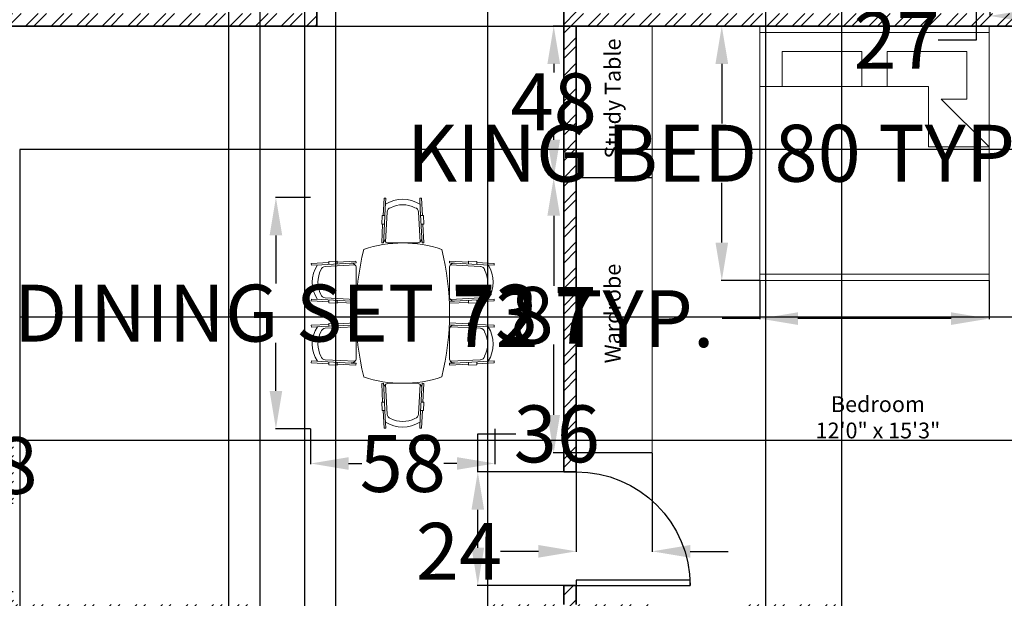
# Model space of a CAD drawing. Units: inches. Extents: x 7 to 752, y -275 to 426.
# Tile 3 of 5: x 284 to 596, y -46 to 137. Entities that reach past the tile are written whole.
import ezdxf

# ---------------------------------------------------------------- set-up
doc = ezdxf.new("R2010")
doc.units = ezdxf.units.IN
for name, color, linetype, lineweight in [('A-ANNO-DIMS', 2, 'Continuous', 18), ('A-ANNO-TEXT', 7, 'Continuous', 18), ('A-AREA-IDEN', 7, 'Continuous', 18), ('A-DOOR', 6, 'Continuous', 25), ('A-FLOR-CASE', 2, 'Continuous', 18), ('A-WALL-PATT', 252, 'Continuous', 13), ('Furniture', 2, 'Continuous', 18), ('Inner Wall', 5, 'Continuous', 35)]:
    doc.layers.add(name, color=color, linetype=linetype, lineweight=lineweight)
doc.styles.get("Standard").update_dxf_attribs({"font": 'arial.ttf'})
doc.dimstyles.get("Standard").update_dxf_attribs({"dimtxt": 18, "dimasz": 12, "dimexe": 0.18, "dimexo": 0.0625, "dimgap": 0.09, "dimtad": 0, "dimtih": 1, "dimtoh": 1, "dimdec": 0, "dimzin": 0, "dimdsep": 46, "dimlunit": 3, "dimtxsty": 'Standard', "dimcen": 0.09, "dimadec": 0, "dimazin": 0, "dimtfac": 1, "dimtdec": 0, "dimtofl": 0, "dimtmove": 0, "dimatfit": 3, "dimfxl": 1, "dimtolj": 1, "dimtzin": 0, "dimarcsym": 0})

# ---------------------------------------------------------------- blocks, each defined once
blk = doc.blocks.new('*U3')
for p, q in [((0, 0), (0, -4)), ((36, 0), (36, -4))]:
    blk.add_line(p, q)
blk.add_lwpolyline([(0, 0), (0, 36), (1.75, 36), (1.75, 0)], close=True)
blk.add_arc((0, 0), 36, 0, 90)
blk = doc.blocks.new('A$C6BEF12A9')
for p, q in [((0.698, 1.955), (0.688, 1.768)), ((0.698, 1.955), (0.718, 1.954)), ((0.718, 1.954), (0.712, 1.841)), ((1.099, 1.955), (1.079, 1.954)), ((1.079, 1.954), (1.085, 1.841)), ((1.099, 1.955), (1.109, 1.768)), ((1.358, 1.955), (1.349, 1.768)), ((1.358, 1.955), (1.378, 1.954)), ((1.378, 1.954), (1.372, 1.841)), ((1.76, 1.955), (1.74, 1.954)), ((1.74, 1.954), (1.746, 1.841)), ((1.76, 1.955), (1.77, 1.768)), ((0.712, 1.841), (0.695, 1.529)), ((0.712, 1.841), (0.695, 1.529)), ((0.73, 1.806), (0.713, 1.488)), ((1.067, 1.806), (1.084, 1.488)), ((1.085, 1.841), (1.102, 1.529)), ((1.372, 1.841), (1.356, 1.529)), ((1.372, 1.841), (1.356, 1.529)), ((1.391, 1.806), (1.374, 1.488)), ((1.728, 1.806), (1.744, 1.488)), ((1.746, 1.841), (1.762, 1.529)), ((0.678, 1.768), (0.673, 1.678)), ((0.708, 1.768), (0.678, 1.768)), ((1.089, 1.768), (1.119, 1.768)), ((1.119, 1.768), (1.124, 1.678)), ((1.339, 1.768), (1.334, 1.678)), ((1.369, 1.768), (1.339, 1.768)), ((1.75, 1.768), (1.78, 1.768)), ((1.78, 1.768), (1.784, 1.678)), ((0.683, 1.678), (0.673, 1.477)), ((0.703, 1.678), (0.673, 1.678)), ((1.094, 1.678), (1.124, 1.678)), ((1.114, 1.678), (1.124, 1.477)), ((1.344, 1.678), (1.333, 1.477)), ((1.364, 1.678), (1.334, 1.678)), ((1.754, 1.678), (1.784, 1.678)), ((1.774, 1.678), (1.785, 1.477)), ((0.673, 1.477), (0.693, 1.476)), ((0.693, 1.476), (0.695, 1.526)), ((0.745, 1.476), (1.052, 1.476)), ((1.104, 1.476), (1.102, 1.526)), ((1.124, 1.477), (1.104, 1.476)), ((1.333, 1.477), (1.353, 1.476)), ((1.353, 1.476), (1.356, 1.526)), ((1.406, 1.476), (1.712, 1.476)), ((1.765, 1.476), (1.762, 1.526)), ((1.785, 1.477), (1.765, 1.476)), ((0, 1.178), (0.187, 1.188)), ((0, 1.178), (0.001, 1.158)), ((0.001, 1.158), (0.114, 1.164)), ((0.114, 1.164), (0.426, 1.181)), ((0.149, 1.146), (0.467, 1.163)), ((0.187, 1.198), (0.277, 1.203)), ((0.187, 1.168), (0.187, 1.198)), ((0.277, 1.193), (0.477, 1.203)), ((0.277, 1.173), (0.277, 1.203)), ((0.479, 1.183), (0.429, 1.181)), ((0.477, 1.203), (0.479, 1.183)), ((1.98, 1.203), (1.979, 1.183)), ((1.979, 1.183), (2.029, 1.181)), ((2.18, 1.193), (1.98, 1.203)), ((2.309, 1.146), (1.99, 1.163)), ((2.343, 1.164), (2.031, 1.181)), ((2.18, 1.173), (2.18, 1.203)), ((2.27, 1.198), (2.18, 1.203)), ((2.27, 1.168), (2.27, 1.198)), ((2.458, 1.178), (2.27, 1.188)), ((2.457, 1.158), (2.343, 1.164)), ((2.458, 1.178), (2.457, 1.158)), ((0.479, 0.824), (0.479, 1.131)), ((1.979, 0.824), (1.979, 1.131)), ((0, 0.777), (0.001, 0.797)), ((0, 0.777), (0.187, 0.767)), ((0.001, 0.797), (0.114, 0.791)), ((0.114, 0.791), (0.426, 0.774)), ((0.114, 0.791), (0.426, 0.774)), ((0.149, 0.809), (0.467, 0.792)), ((0.187, 0.787), (0.187, 0.757)), ((0.187, 0.757), (0.277, 0.752)), ((0.277, 0.782), (0.277, 0.752)), ((0.277, 0.762), (0.477, 0.752)), ((0.479, 0.772), (0.429, 0.774)), ((0.477, 0.752), (0.479, 0.772)), ((1.979, 0.772), (2.029, 0.774)), ((1.98, 0.752), (1.979, 0.772)), ((2.18, 0.762), (1.98, 0.752)), ((2.309, 0.809), (1.99, 0.792)), ((2.343, 0.791), (2.031, 0.774)), ((2.343, 0.791), (2.031, 0.774)), ((2.18, 0.782), (2.18, 0.752)), ((2.27, 0.757), (2.18, 0.752)), ((2.27, 0.787), (2.27, 0.757)), ((2.458, 0.777), (2.27, 0.767)), ((2.457, 0.797), (2.343, 0.791)), ((2.458, 0.777), (2.457, 0.797)), ((0.673, 0.477), (0.693, 0.479)), ((0.683, 0.277), (0.673, 0.477)), ((0.693, 0.479), (0.695, 0.429)), ((0.712, 0.114), (0.695, 0.426)), ((0.712, 0.114), (0.695, 0.426)), ((0.73, 0.149), (0.713, 0.467)), ((0.745, 0.479), (1.052, 0.479)), ((1.067, 0.149), (1.084, 0.467)), ((1.085, 0.114), (1.102, 0.426)), ((1.104, 0.479), (1.102, 0.429)), ((1.124, 0.477), (1.104, 0.479)), ((1.114, 0.277), (1.124, 0.477)), ((1.333, 0.477), (1.353, 0.479)), ((1.344, 0.277), (1.333, 0.477)), ((1.353, 0.479), (1.356, 0.429)), ((1.372, 0.114), (1.356, 0.426)), ((1.372, 0.114), (1.356, 0.426)), ((1.391, 0.149), (1.374, 0.467)), ((1.406, 0.479), (1.712, 0.479)), ((1.728, 0.149), (1.744, 0.467)), ((1.746, 0.114), (1.762, 0.426)), ((1.765, 0.479), (1.762, 0.429)), ((1.785, 0.477), (1.765, 0.479)), ((1.774, 0.277), (1.785, 0.477)), ((0.678, 0.187), (0.673, 0.277)), ((0.703, 0.277), (0.673, 0.277)), ((1.094, 0.277), (1.124, 0.277)), ((1.119, 0.187), (1.124, 0.277)), ((1.364, 0.277), (1.334, 0.277)), ((1.339, 0.187), (1.334, 0.277)), ((1.754, 0.277), (1.784, 0.277)), ((1.78, 0.187), (1.784, 0.277)), ((0.708, 0.187), (0.678, 0.187)), ((0.698, 0), (0.688, 0.187)), ((0.718, 0.001), (0.712, 0.114)), ((1.079, 0.001), (1.085, 0.114)), ((1.089, 0.187), (1.119, 0.187)), ((1.099, 0), (1.109, 0.187)), ((1.369, 0.187), (1.339, 0.187)), ((1.358, 0), (1.349, 0.187)), ((1.378, 0.001), (1.372, 0.114)), ((1.74, 0.001), (1.746, 0.114)), ((1.75, 0.187), (1.78, 0.187)), ((1.76, 0), (1.77, 0.187)), ((0.698, 0), (0.718, 0.001)), ((1.099, 0), (1.079, 0.001)), ((1.358, 0), (1.378, 0.001)), ((1.76, 0), (1.74, 0.001))]:
    blk.add_line(p, q)
for centre, radius, start, end in [((0.898, 1.603), 0.341, 57.3412, 122.6588), ((1.559, 1.603), 0.341, 57.3412, 122.6588), ((0.78, 1.804), 0.05, 103.7138, 177), ((0.898, 1.603), 0.281, 62.3651, 117.6349), ((1.017, 1.804), 0.05, 3, 76.2862), ((1.441, 1.804), 0.05, 103.7138, 177), ((1.559, 1.603), 0.281, 62.3651, 117.6349), ((1.678, 1.804), 0.05, 3, 76.2862), ((1.229, -1.385), 2.862, 76.2365, 103.7635), ((0.745, 1.526), 0.05, 177, 270), ((1.052, 1.526), 0.05, 270, 3), ((1.406, 1.526), 0.05, 177, 270), ((1.712, 1.526), 0.05, 270, 3), ((1.779, 0.977), 1.3, 161.253, 198.747), ((0.679, 0.977), 1.3, 341.253, 18.747), ((0.352, 0.977), 0.341, 147.3412, 212.6588), ((0.429, 1.131), 0.05, 0, 93), ((2.029, 1.131), 0.05, 87, 180), ((2.106, 0.977), 0.341, 327.3412, 32.6588), ((0.352, 0.977), 0.281, 152.3651, 207.6349), ((0.151, 1.096), 0.05, 93, 166.2862), ((2.306, 1.096), 0.05, 13.7138, 87), ((2.106, 0.977), 0.281, 332.3651, 27.6349), ((0.151, 0.859), 0.05, 193.7138, 267), ((2.306, 0.859), 0.05, 273, 346.2862), ((0.429, 0.824), 0.05, 267, 0), ((2.029, 0.824), 0.05, 180, 273), ((1.229, 3.34), 2.862, 256.2365, 283.7635), ((0.745, 0.429), 0.05, 90, 183), ((1.052, 0.429), 0.05, 357, 90), ((1.406, 0.429), 0.05, 90, 183), ((1.712, 0.429), 0.05, 357, 90), ((0.78, 0.151), 0.05, 183, 256.2862), ((1.017, 0.151), 0.05, 283.7138, 357), ((1.441, 0.151), 0.05, 183, 256.2862), ((1.678, 0.151), 0.05, 283.7138, 357), ((0.898, 0.352), 0.341, 237.3412, 302.6588), ((0.898, 0.352), 0.281, 242.3651, 297.6349), ((1.559, 0.352), 0.341, 237.3412, 302.6588), ((1.559, 0.352), 0.281, 242.3651, 297.6349)]:
    blk.add_arc(centre, radius, start, end)
blk = doc.blocks.new('KING-00')
for p, q in [((-0.8967, -0.947), (-0.8967, 0.8818)), ((0.6019, 0.8818), (0.6019, -0.4644)), ((1.0337, -0.947), (1.0337, 0.8818)), ((0.6019, 0.704), (0.8813, 0.704)), ((0.8813, 0.069), (0.8813, 0.704)), ((0.6019, 0.069), (0.8813, 0.069)), ((0.8813, -0.1342), (0.6019, -0.1342)), ((0.8813, -0.7692), (0.8813, -0.1342)), ((0.1193, -0.4644), (0.1193, -0.947)), ((0.6019, -0.4644), (0.1193, -0.4644)), ((0.1193, -0.947), (0.5003, -0.566)), ((0.5003, -0.7692), (0.5003, -0.566)), ((0.5003, -0.7692), (0.8813, -0.7692))]:
    blk.add_line(p, q)
blk.add_lwpolyline([(-0.9475, -0.947), (-0.9475, 0.8818), (1.0845, 0.8818), (1.0845, -0.947)], close=True)
blk = doc.blocks.new('*D20')
at = {"layer": 'A-ANNO-DIMS', "color": 0, "lineweight": -2, "transparency": 16777216}
for p, q in [((518.33, 134.68), (506.15, 134.68)), ((506.33, 122.68), (506.33, 103.84)), ((506.33, 66.2), (506.33, 85.04)), ((518.33, 54.2), (506.15, 54.2))]:
    blk.add_line(p, q, dxfattribs=at)
at = {"layer": 'A-ANNO-DIMS', "color": 0, "transparency": 16777216}
for points in [[(504.33, 122.68), (508.33, 122.68), (506.33, 134.68)], [(504.33, 66.2), (508.33, 66.2), (506.33, 54.2)]]:
    blk.add_solid(points, dxfattribs=at)
at = {"layer": 'Defpoints', "color": 0, "transparency": 16777216}
for p in [(506.33, 134.68), (518.4, 134.68), (518.4, 54.2)]:
    blk.add_point(p, dxfattribs=at)
at = {"layer": 'A-ANNO-DIMS', "color": 0, "transparency": 16777216, "insert": (506.33, 94.44), "char_height": 18, "attachment_point": 5}
blk.add_mtext('\\A1;KING BED 80 TYP.', dxfattribs=at)
blk = doc.blocks.new('*D21')
at = {"layer": 'A-ANNO-DIMS', "color": 0, "lineweight": -2, "transparency": 16777216}
for p, q in [((518.4, 54.14), (518.4, 41.95)), ((590.82, 54.14), (590.82, 41.95)), ((518.4, 42.13), (506.4, 42.13)), ((578.82, 42.13), (530.4, 42.13))]:
    blk.add_line(p, q, dxfattribs=at)
at = {"layer": 'A-ANNO-DIMS', "color": 0, "transparency": 16777216}
for points in [[(530.4, 44.13), (530.4, 40.13), (518.4, 42.13)], [(578.82, 44.13), (578.82, 40.13), (590.82, 42.13)]]:
    blk.add_solid(points, dxfattribs=at)
at = {"layer": 'Defpoints', "color": 0, "transparency": 16777216}
for p in [(518.4, 54.2), (590.82, 54.2), (518.4, 42.13)]:
    blk.add_point(p, dxfattribs=at)
at = {"layer": 'A-ANNO-DIMS', "color": 0, "transparency": 16777216, "insert": (462.57, 42.13), "char_height": 18, "attachment_point": 5}
blk.add_mtext('\\A1;72 TYP.', dxfattribs=at)
blk = doc.blocks.new('*D22')
at = {"layer": 'A-ANNO-DIMS', "color": 0, "lineweight": -2, "transparency": 16777216}
for p, q in [((376.25, 80.45), (365.16, 80.45)), ((365.34, 68.45), (365.34, 53.28)), ((365.34, 19.29), (365.34, 34.47)), ((376.25, 7.29), (365.16, 7.29))]:
    blk.add_line(p, q, dxfattribs=at)
at = {"layer": 'A-ANNO-DIMS', "color": 0, "transparency": 16777216}
for points in [[(363.34, 68.45), (367.34, 68.45), (365.34, 80.45)], [(363.34, 19.29), (367.34, 19.29), (365.34, 7.29)]]:
    blk.add_solid(points, dxfattribs=at)
at = {"layer": 'Defpoints', "color": 0, "transparency": 16777216}
for p in [(376.32, 80.45), (365.34, 7.29), (376.32, 7.29)]:
    blk.add_point(p, dxfattribs=at)
at = {"layer": 'A-ANNO-DIMS', "color": 0, "transparency": 16777216, "insert": (365.34, 43.87), "char_height": 18, "attachment_point": 5}
blk.add_mtext('\\A1;DINING SET 73', dxfattribs=at)
blk = doc.blocks.new('*D23')
at = {"layer": 'A-ANNO-DIMS', "color": 0, "lineweight": -2, "transparency": 16777216}
for p, q in [((376.32, 7.23), (376.32, -3.86)), ((434.6, 7.23), (434.6, -3.86)), ((388.32, -3.68), (392.46, -3.68)), ((422.6, -3.68), (418.46, -3.68))]:
    blk.add_line(p, q, dxfattribs=at)
at = {"layer": 'A-ANNO-DIMS', "color": 0, "transparency": 16777216}
for points in [[(388.32, -1.68), (388.32, -5.68), (376.32, -3.68)], [(422.6, -1.68), (422.6, -5.68), (434.6, -3.68)]]:
    blk.add_solid(points, dxfattribs=at)
at = {"layer": 'Defpoints', "color": 0, "transparency": 16777216}
for p in [(376.32, 7.29), (434.6, 7.29), (434.6, -3.68)]:
    blk.add_point(p, dxfattribs=at)
at = {"layer": 'A-ANNO-DIMS', "color": 0, "transparency": 16777216, "insert": (405.46, -3.68), "char_height": 18, "attachment_point": 5}
blk.add_mtext('\\A1;58', dxfattribs=at)
blk = doc.blocks.new('*D26')
at = {"layer": 'A-ANNO-DIMS', "color": 0, "lineweight": -2, "transparency": 16777216}
for p, q in [((591.04, 142.1), (591.04, 137.69)), ((619.61, 142.1), (619.61, 137.69)), ((603.04, 137.87), (607.61, 137.87)), ((619.61, 137.87), (631.61, 137.87))]:
    blk.add_line(p, q, dxfattribs=at)
at = {"layer": 'A-ANNO-DIMS', "color": 0, "transparency": 16777216}
for points in [[(603.04, 139.87), (603.04, 135.87), (591.04, 137.87)], [(607.61, 139.87), (607.61, 135.87), (619.61, 137.87)]]:
    blk.add_solid(points, dxfattribs=at)
at = {"layer": 'Defpoints', "color": 0, "transparency": 16777216}
for p in [(591.04, 142.16), (619.61, 142.16), (619.61, 137.87)]:
    blk.add_point(p, dxfattribs=at)
at = {"layer": 'A-ANNO-DIMS', "color": 0, "transparency": 16777216, "insert": (695.1, 137.87), "char_height": 18, "attachment_point": 5}
blk.add_mtext('\\A1;FRIDGE 29', dxfattribs=at)
blk = doc.blocks.new('*D27')
at = {"layer": 'A-ANNO-DIMS', "color": 0, "lineweight": -2, "transparency": 16777216}
for p, q in [((590.98, 168.83), (586.58, 168.83)), ((586.76, 156.83), (586.76, 154.16)), ((590.98, 142.16), (586.58, 142.16)), ((586.76, 142.16), (586.76, 130.16)), ((586.76, 130.16), (574.76, 130.16))]:
    blk.add_line(p, q, dxfattribs=at)
at = {"layer": 'A-ANNO-DIMS', "color": 0, "transparency": 16777216}
for points in [[(584.76, 156.83), (588.76, 156.83), (586.76, 168.83)], [(584.76, 154.16), (588.76, 154.16), (586.76, 142.16)]]:
    blk.add_solid(points, dxfattribs=at)
at = {"layer": 'Defpoints', "color": 0, "transparency": 16777216}
for p in [(591.04, 168.83), (586.76, 142.16), (591.04, 142.16)]:
    blk.add_point(p, dxfattribs=at)
at = {"layer": 'A-ANNO-DIMS', "color": 0, "transparency": 16777216, "insert": (561.62, 130.16), "char_height": 18, "attachment_point": 5}
blk.add_mtext('\\A1;27', dxfattribs=at)
blk = doc.blocks.new('*D39')
at = {"layer": 'A-ANNO-DIMS', "color": 0, "lineweight": -2, "transparency": 16777216}
for p, q in [((348.33, 413.83), (336.33, 413.83)), ((360.33, -131.26), (360.33, 414.01)), ((384.33, -131.26), (384.33, 414.01)), ((396.33, 413.83), (408.33, 413.83))]:
    blk.add_line(p, q, dxfattribs=at)
at = {"layer": 'A-ANNO-DIMS', "color": 0, "transparency": 16777216}
for points in [[(348.33, 415.83), (348.33, 411.83), (360.33, 413.83)], [(396.33, 415.83), (396.33, 411.83), (384.33, 413.83)]]:
    blk.add_solid(points, dxfattribs=at)
at = {"layer": 'Defpoints', "color": 0, "transparency": 16777216}
for p in [(384.33, 413.83), (360.33, -131.32), (384.33, -131.32)]:
    blk.add_point(p, dxfattribs=at)
at = {"layer": 'A-ANNO-DIMS', "color": 0, "transparency": 16777216, "insert": (421.43, 413.83), "char_height": 18, "attachment_point": 5}
blk.add_mtext('\\A1;24', dxfattribs=at)
blk = doc.blocks.new('*D40')
at = {"layer": 'A-ANNO-DIMS', "color": 0, "lineweight": -2, "transparency": 16777216}
for p, q in [((372.328243, 413.826615), (360.328243, 413.826615)), ((384.328243, -106.961989), (384.328243, 414.006615)), ((432.328243, -106.961989), (432.328243, 414.006615)), ((444.328243, 413.826615), (456.328243, 413.826615))]:
    blk.add_line(p, q, dxfattribs=at)
at = {"layer": 'A-ANNO-DIMS', "color": 0, "transparency": 16777216}
for points in [[(372.328243, 415.826615), (372.328243, 411.826615), (384.328243, 413.826615)], [(444.328243, 415.826615), (444.328243, 411.826615), (432.328243, 413.826615)]]:
    blk.add_solid(points, dxfattribs=at)
at = {"layer": 'Defpoints', "color": 0, "transparency": 16777216}
for p in [(432.328243, 413.826615), (384.328243, -107.024489), (432.328243, -107.024489)]:
    blk.add_point(p, dxfattribs=at)
at = {"layer": 'A-ANNO-DIMS', "color": 0, "transparency": 16777216, "insert": (408.328243, 413.826615), "char_height": 18, "attachment_point": 5}
blk.add_mtext('\\A1;48', dxfattribs=at)
blk = doc.blocks.new('*D42')
at = {"layer": 'A-ANNO-DIMS', "color": 0, "lineweight": -2, "transparency": 16777216}
for p, q in [((221.33, 95.61), (221.33, -259.65)), ((284.33, 95.61), (284.33, -259.65)), ((233.33, -259.47), (239.8, -259.47)), ((272.33, -259.47), (265.86, -259.47))]:
    blk.add_line(p, q, dxfattribs=at)
at = {"layer": 'A-ANNO-DIMS', "color": 0, "transparency": 16777216}
for points in [[(233.33, -257.47), (233.33, -261.47), (221.33, -259.47)], [(272.33, -257.47), (272.33, -261.47), (284.33, -259.47)]]:
    blk.add_solid(points, dxfattribs=at)
at = {"layer": 'Defpoints', "color": 0, "transparency": 16777216}
for p in [(221.33, 95.68), (284.33, 95.68), (284.33, -259.47)]:
    blk.add_point(p, dxfattribs=at)
at = {"layer": 'A-ANNO-DIMS', "color": 0, "transparency": 16777216, "insert": (252.83, -259.47), "char_height": 18, "attachment_point": 5}
blk.add_mtext('\\A1;63', dxfattribs=at)
blk = doc.blocks.new('*D43')
at = {"layer": 'A-ANNO-DIMS', "color": 0, "lineweight": -2, "transparency": 16777216}
for p, q in [((221.39, 134.68), (657.66, 134.68)), ((657.48, 122.68), (657.48, 78.46)), ((657.48, 15.68), (657.48, 59.89)), ((221.39, 3.68), (657.66, 3.68))]:
    blk.add_line(p, q, dxfattribs=at)
at = {"layer": 'A-ANNO-DIMS', "color": 0, "transparency": 16777216}
for points in [[(655.48, 122.68), (659.48, 122.68), (657.48, 134.68)], [(655.48, 15.68), (659.48, 15.68), (657.48, 3.68)]]:
    blk.add_solid(points, dxfattribs=at)
at = {"layer": 'Defpoints', "color": 0, "transparency": 16777216}
for p in [(221.33, 134.68), (657.48, 134.68), (221.33, 3.68)]:
    blk.add_point(p, dxfattribs=at)
at = {"layer": 'A-ANNO-DIMS', "color": 0, "transparency": 16777216, "insert": (657.48, 69.18), "char_height": 18, "attachment_point": 5}
blk.add_mtext('\\A1;131', dxfattribs=at)
blk = doc.blocks.new('*D44')
at = {"layer": 'A-ANNO-DIMS', "color": 0, "lineweight": -2, "transparency": 16777216}
for p, q in [((657.48, 42.68), (657.48, 54.68)), ((657.48, 54.68), (669.48, 54.68)), ((284.39, 42.68), (657.66, 42.68)), ((657.48, 15.68), (657.48, 30.68)), ((284.39, 3.68), (657.66, 3.68))]:
    blk.add_line(p, q, dxfattribs=at)
at = {"layer": 'A-ANNO-DIMS', "color": 0, "transparency": 16777216}
for points in [[(655.48, 30.68), (659.48, 30.68), (657.48, 42.68)], [(655.48, 15.68), (659.48, 15.68), (657.48, 3.68)]]:
    blk.add_solid(points, dxfattribs=at)
at = {"layer": 'Defpoints', "color": 0, "transparency": 16777216}
for p in [(284.33, 42.68), (657.48, 42.68), (284.33, 3.68)]:
    blk.add_point(p, dxfattribs=at)
at = {"layer": 'A-ANNO-DIMS', "color": 0, "transparency": 16777216, "insert": (682.47, 54.68), "char_height": 18, "attachment_point": 5}
blk.add_mtext('\\A1;39', dxfattribs=at)
blk = doc.blocks.new('*D45')
at = {"layer": 'A-ANNO-DIMS', "color": 0, "lineweight": -2, "transparency": 16777216}
for p, q in [((284.39, 95.68), (657.66, 95.68)), ((657.48, 83.68), (657.48, 78.46)), ((657.48, 54.68), (657.48, 59.89)), ((284.39, 42.68), (657.66, 42.68))]:
    blk.add_line(p, q, dxfattribs=at)
at = {"layer": 'A-ANNO-DIMS', "color": 0, "transparency": 16777216}
for points in [[(655.48, 83.68), (659.48, 83.68), (657.48, 95.68)], [(655.48, 54.68), (659.48, 54.68), (657.48, 42.68)]]:
    blk.add_solid(points, dxfattribs=at)
at = {"layer": 'Defpoints', "color": 0, "transparency": 16777216}
for p in [(284.33, 95.68), (657.48, 95.68), (284.33, 42.68)]:
    blk.add_point(p, dxfattribs=at)
at = {"layer": 'A-ANNO-DIMS', "color": 0, "transparency": 16777216, "insert": (657.48, 69.18), "char_height": 18, "attachment_point": 5}
blk.add_mtext('\\A1;53', dxfattribs=at)
blk = doc.blocks.new('*D46')
at = {"layer": 'A-ANNO-DIMS', "color": 0, "lineweight": -2, "transparency": 16777216}
for p, q in [((520.16, 197.44), (520.16, -259.65)), ((544.16, 197.44), (544.16, -259.65)), ((508.16, -259.47), (496.16, -259.47)), ((556.16, -259.47), (568.16, -259.47))]:
    blk.add_line(p, q, dxfattribs=at)
at = {"layer": 'A-ANNO-DIMS', "color": 0, "transparency": 16777216}
for points in [[(508.16, -257.47), (508.16, -261.47), (520.16, -259.47)], [(556.16, -257.47), (556.16, -261.47), (544.16, -259.47)]]:
    blk.add_solid(points, dxfattribs=at)
at = {"layer": 'Defpoints', "color": 0, "transparency": 16777216}
for p in [(520.16, 197.5), (544.16, 197.5), (544.16, -259.47)]:
    blk.add_point(p, dxfattribs=at)
at = {"layer": 'A-ANNO-DIMS', "color": 0, "transparency": 16777216, "insert": (581.26, -259.47), "char_height": 18, "attachment_point": 5}
blk.add_mtext('\\A1;24', dxfattribs=at)
blk = doc.blocks.new('*D52')
at = {"layer": 'A-ANNO-DIMS', "color": 0, "lineweight": -2, "transparency": 16777216}
for p, q in [((350.33, 198.78), (350.33, -259.65)), ((374.33, 198.78), (374.33, -259.65)), ((338.33, -259.47), (326.33, -259.47)), ((386.33, -259.47), (398.33, -259.47))]:
    blk.add_line(p, q, dxfattribs=at)
at = {"layer": 'A-ANNO-DIMS', "color": 0, "transparency": 16777216}
for points in [[(338.33, -257.47), (338.33, -261.47), (350.33, -259.47)], [(386.33, -257.47), (386.33, -261.47), (374.33, -259.47)]]:
    blk.add_solid(points, dxfattribs=at)
at = {"layer": 'Defpoints', "color": 0, "transparency": 16777216}
for p in [(350.33, 198.85), (374.33, 198.85), (374.33, -259.47)]:
    blk.add_point(p, dxfattribs=at)
at = {"layer": 'A-ANNO-DIMS', "color": 0, "transparency": 16777216, "insert": (411.43, -259.47), "char_height": 18, "attachment_point": 5}
blk.add_mtext('\\A1;24', dxfattribs=at)
blk = doc.blocks.new('*D55')
at = {"layer": 'A-ANNO-DIMS', "color": 0, "lineweight": -2, "transparency": 16777216}
for p, q in [((429.18, -6.32), (429.18, 5.68)), ((429.18, 5.68), (441.18, 5.68)), ((460.27, -6.32), (429, -6.32)), ((429.18, -30.32), (429.18, -18.32)), ((460.27, -42.32), (429, -42.32))]:
    blk.add_line(p, q, dxfattribs=at)
at = {"layer": 'A-ANNO-DIMS', "color": 0, "transparency": 16777216}
for points in [[(427.18, -18.32), (431.18, -18.32), (429.18, -6.32)], [(427.18, -30.32), (431.18, -30.32), (429.18, -42.32)]]:
    blk.add_solid(points, dxfattribs=at)
at = {"layer": 'Defpoints', "color": 0, "transparency": 16777216}
for p in [(429.18, -6.32), (460.33, -6.32), (460.33, -42.32)]:
    blk.add_point(p, dxfattribs=at)
at = {"layer": 'A-ANNO-DIMS', "color": 0, "transparency": 16777216, "insert": (454.15, 5.68), "char_height": 18, "attachment_point": 5}
blk.add_mtext('\\A1;36', dxfattribs=at)
blk = doc.blocks.new('*D57')
at = {"layer": 'A-ANNO-DIMS', "color": 0, "lineweight": -2, "transparency": 16777216}
for p, q in [((460.33, -0.39), (460.33, -31.65)), ((484.33, -0.39), (484.33, -31.65)), ((448.33, -31.47), (436.33, -31.47)), ((496.33, -31.47), (508.33, -31.47))]:
    blk.add_line(p, q, dxfattribs=at)
at = {"layer": 'A-ANNO-DIMS', "color": 0, "transparency": 16777216}
for points in [[(448.33, -29.47), (448.33, -33.47), (460.33, -31.47)], [(496.33, -29.47), (496.33, -33.47), (484.33, -31.47)]]:
    blk.add_solid(points, dxfattribs=at)
at = {"layer": 'Defpoints', "color": 0, "transparency": 16777216}
for p in [(460.33, -0.32), (484.33, -0.32), (460.33, -31.47)]:
    blk.add_point(p, dxfattribs=at)
at = {"layer": 'A-ANNO-DIMS', "color": 0, "transparency": 16777216, "insert": (423.23, -31.47), "char_height": 18, "attachment_point": 5}
blk.add_mtext('\\A1;24', dxfattribs=at)
blk = doc.blocks.new('*D58')
at = {"layer": 'A-ANNO-DIMS', "color": 0, "lineweight": -2, "transparency": 16777216}
for p, q in [((484.27, 86.68), (453, 86.68)), ((453.18, 74.68), (453.18, 52.46)), ((453.18, 11.68), (453.18, 33.9)), ((484.27, -0.32), (453, -0.32))]:
    blk.add_line(p, q, dxfattribs=at)
at = {"layer": 'A-ANNO-DIMS', "color": 0, "transparency": 16777216}
for points in [[(451.18, 74.68), (455.18, 74.68), (453.18, 86.68)], [(451.18, 11.68), (455.18, 11.68), (453.18, -0.32)]]:
    blk.add_solid(points, dxfattribs=at)
at = {"layer": 'Defpoints', "color": 0, "transparency": 16777216}
for p in [(453.18, 86.68), (484.33, 86.68), (484.33, -0.32)]:
    blk.add_point(p, dxfattribs=at)
at = {"layer": 'A-ANNO-DIMS', "color": 0, "transparency": 16777216, "insert": (453.18, 43.18), "char_height": 18, "attachment_point": 5}
blk.add_mtext('\\A1;87', dxfattribs=at)
blk = doc.blocks.new('*D59')
at = {"layer": 'A-ANNO-DIMS', "color": 0, "lineweight": -2, "transparency": 16777216}
for p, q in [((484.27, 134.68), (453, 134.68)), ((453.18, 122.68), (453.18, 119.96)), ((453.18, 98.68), (453.18, 101.4)), ((484.27, 86.68), (453, 86.68))]:
    blk.add_line(p, q, dxfattribs=at)
at = {"layer": 'A-ANNO-DIMS', "color": 0, "transparency": 16777216}
for points in [[(451.18, 122.68), (455.18, 122.68), (453.18, 134.68)], [(451.18, 98.68), (455.18, 98.68), (453.18, 86.68)]]:
    blk.add_solid(points, dxfattribs=at)
at = {"layer": 'Defpoints', "color": 0, "transparency": 16777216}
for p in [(453.18, 134.68), (484.33, 134.68), (484.33, 86.68)]:
    blk.add_point(p, dxfattribs=at)
at = {"layer": 'A-ANNO-DIMS', "color": 0, "transparency": 16777216, "insert": (453.18, 110.68), "char_height": 18, "attachment_point": 5}
blk.add_mtext('\\A1;48', dxfattribs=at)
blk = doc.blocks.new('*D63')
at = {"layer": 'A-ANNO-DIMS', "color": 0, "lineweight": -2, "transparency": 16777216}
for p, q in [((251.18, -16.32), (251.18, -4.32)), ((251.18, -4.32), (263.18, -4.32)), ((282.27, -16.32), (251, -16.32)), ((251.18, -32.32), (251.18, -28.32)), ((282.27, -44.32), (251, -44.32))]:
    blk.add_line(p, q, dxfattribs=at)
at = {"layer": 'A-ANNO-DIMS', "color": 0, "transparency": 16777216}
for points in [[(249.18, -28.32), (253.18, -28.32), (251.18, -16.32)], [(249.18, -32.32), (253.18, -32.32), (251.18, -44.32)]]:
    blk.add_solid(points, dxfattribs=at)
at = {"layer": 'Defpoints', "color": 0, "transparency": 16777216}
for p in [(251.18, -16.32), (282.33, -16.32), (282.33, -44.32)]:
    blk.add_point(p, dxfattribs=at)
at = {"layer": 'A-ANNO-DIMS', "color": 0, "transparency": 16777216, "insert": (276.33, -4.32), "char_height": 18, "attachment_point": 5}
blk.add_mtext('\\A1;28', dxfattribs=at)

msp = doc.modelspace()

# ---------------------------------------------------------------- hatches: boundary and pattern name
at = {"layer": 'A-WALL-PATT'}
h = msp.add_hatch(dxfattribs=at)
h.set_pattern_fill('ANSI32', color=256, scale=0.6)
h.set_pattern_definition([(45, (-434.707, -1257.0093), (-4.041115, 4.041115), []), (45, (-432.013, -1257.0093), (-4.041115, 4.041115), [])])
h.paths.add_polyline_path([(360.33, -48.32), (282.33, -48.32), (282.33, -44.32), (278.33, -44.32), (278.33, -48.32), (182.33, -48.32), (182.33, -54.32), (356.33, -54.32), (356.33, -89.32), (360.33, -89.32)])
h.paths.add_polyline_path([(484.33, -48.32), (460.33, -48.32), (460.33, -42.32), (456.33, -42.32), (456.33, -48.32), (432.33, -48.32), (432.33, -52.32), (456.33, -52.32), (456.33, -131.32), (460.33, -131.32), (460.33, -52.32), (484.33, -52.32)])
h.paths.add_polyline_path([(544.33, -48.32), (512.33, -48.32), (512.33, -52.32), (544.33, -52.32)])
h.paths.add_polyline_path([(460.33, 134.68), (484.33, 134.68), (620.33, 134.68), (620.33, 138.68), (460.33, 138.68), (460.33, 144.68), (456.33, 144.68), (456.33, -6.32), (460.33, -6.32)])
h.paths.add_polyline_path([(282.33, 3.68), (182.33, 3.68), (182.33, -0.32), (278.33, -0.32), (278.33, -16.32), (282.33, -16.32)])
h.paths.add_polyline_path([(378.33, 144.68), (374.33, 144.68), (374.33, 138.68), (182.33, 138.68), (182.33, 134.68), (378.33, 134.68)])
h.paths.add_polyline_path([(284.33, 306.68), (278.33, 306.68), (278.33, 286.68), (240.33, 286.68), (240.33, 282.68), (284.33, 282.68)])
h.paths.add_polyline_path([(212.33, 286.68), (182.33, 286.68), (182.33, 282.68), (212.33, 282.68)])
h.paths.add_polyline_path([(436.33, 225.08), (460.33, 225.08), (460.33, 229.08), (432.33, 229.08), (432.33, 184.68), (456.33, 184.68), (456.33, 180.68), (460.33, 180.68), (460.33, 188.68), (436.33, 188.68)])
h.paths.add_polyline_path([(432.33, 204.68), (378.33, 204.68), (378.33, 306.68), (374.33, 306.68), (374.33, 282.68), (374.33, 198.85), (374.33, 180.68), (378.33, 180.68), (378.33, 200.68), (432.33, 200.68)])
h.paths.add_polyline_path([(460.33, 270.68), (436.33, 270.68), (436.33, 306.68), (432.33, 306.68), (432.33, 282.68), (432.33, 266.68), (460.33, 266.68)])

# ---------------------------------------------------------------- linework, layer by layer
at = {"layer": 'A-FLOR-CASE'}
for points in [[(460.33, 134.68), (484.33, 134.68), (484.33, 86.68), (460.33, 86.68)], [(460.33, 86.68), (484.33, 86.68), (484.33, -0.32), (460.33, -0.32)]]:
    msp.add_lwpolyline(points, close=True, dxfattribs=at)
at = {"layer": 'Inner Wall'}
for p, q in [((378.33, 144.68), (378.33, 134.68)), ((456.33, 144.68), (456.33, -6.32)), ((182.33, 134.68), (378.33, 134.68)), ((460.33, 134.68), (620.33, 134.68)), ((460.33, 134.68), (460.33, -6.32)), ((456.33, -6.32), (460.33, -6.32)), ((456.33, -42.32), (460.33, -42.32)), ((456.33, -42.32), (456.33, -48.32)), ((460.33, -42.32), (460.33, -48.32))]:
    msp.add_line(p, q, dxfattribs=at)

# ---------------------------------------------------------------- block references
at = {"layer": 'A-DOOR', "xscale": -1, "rotation": 270}
msp.add_blockref('*U3', (460.33, -42.32), dxfattribs=at)
at = {"layer": 'Furniture'}
for name, p, xscale, yscale, zscale, rotation in [('KING-00', (553.32, 91.73), 39.60249106241186, 39.60249106241186, 39.60249106241186, 90), ('A$C6BEF12A9', (376.53, 80.24), 29.59247402267948, 29.59247402267948, 29.59247402267948, 270)]:
    msp.add_blockref(name, p, dxfattribs=dict(at, xscale=xscale, yscale=yscale, zscale=zscale, rotation=rotation))

# ---------------------------------------------------------------- texts
at = {"layer": 'A-ANNO-TEXT', "char_height": 5, "attachment_point": 3, "rotation": 90}
for s, insert in [('\\pxqc;{\\fTimes New Roman|b0|i0|c0|p18;Study Table}', (469.34, 136.29)), ('\\pxqc;{\\fTimes New Roman|b0|i0|c0|p18;Wardrobe}', (469.34, 68.29))]:
    msp.add_mtext_dynamic_manual_height_columns(s, width=49.1019, gutter_width=12.5, heights=[0], dxfattribs=dict(at, insert=insert))
at = {"layer": 'A-AREA-IDEN', "insert": (580.25, 17.59), "char_height": 5, "attachment_point": 3}
msp.add_mtext_dynamic_manual_height_columns('\\pxqc;{\\fTimes New Roman|b0|i0|c0|p18;Bedroom\\P12\'0" x 15\'3"}', width=49.1019, gutter_width=12.5, heights=[0], dxfattribs=at)

# ---------------------------------------------------------------- dimensions: what is measured, and where the dimension line sits
at = {"layer": 'A-ANNO-DIMS'}
for base, p1, p2, picture, middle in [((384.33, 413.83), (360.33, -131.32), (384.33, -131.32), '*D39', (421.43, 413.83)), ((432.33, 413.83), (384.33, -107.02), (432.33, -107.02), '*D40', (408.33, 413.83)), ((374.33, -259.47), (350.33, 198.85), (374.33, 198.85), '*D52', (411.43, -259.47)), ((544.16, -259.47), (520.16, 197.5), (544.16, 197.5), '*D46', (581.26, -259.47)), ((284.33, -259.47), (221.33, 95.68), (284.33, 95.68), '*D42', (252.83, -259.47)), ((434.6, -3.68), (376.32, 7.29), (434.6, 7.29), '*D23', (405.46, -3.68))]:
    dim = msp.add_linear_dim(base=base, p1=p1, p2=p2, dimstyle='Standard', override={"dimdec": 0, "dimlfac": 1, "dimrnd": 0, "dimzin": 0, "dimdsep": 46, "dimlunit": 2}, dxfattribs=at)
    dim.commit()
    dim.dimension.update_dxf_attribs({"geometry": picture, "text_midpoint": middle})
for base, p1, p2, angle, picture, middle in [((586.76, 142.16), (591.04, 168.83), (591.04, 142.16), 270, '*D27', (561.62, 130.16)), ((657.48, 134.68), (221.33, 3.68), (221.33, 134.68), 90, '*D43', (657.48, 69.18)), ((453.18, 134.68), (484.33, 86.68), (484.33, 134.68), 90, '*D59', (453.18, 110.68)), ((657.48, 95.68), (284.33, 42.68), (284.33, 95.68), 90, '*D45', (657.48, 69.18)), ((453.18, 86.68), (484.33, -0.32), (484.33, 86.68), 90, '*D58', (453.18, 43.18)), ((657.48, 42.68), (284.33, 3.68), (284.33, 42.68), 90, '*D44', (682.47, 54.68)), ((429.18, -6.32), (460.33, -42.32), (460.33, -6.32), 90, '*D55', (454.15, 5.68)), ((251.18, -16.32), (282.33, -44.32), (282.33, -16.32), 90, '*D63', (276.33, -4.32)), ((460.33, -31.47), (484.33, -0.32), (460.33, -0.32), 180, '*D57', (423.23, -31.47))]:
    dim = msp.add_linear_dim(base=base, p1=p1, p2=p2, angle=angle, dimstyle='Standard', override={"dimdec": 0, "dimlfac": 1, "dimrnd": 0, "dimzin": 0, "dimdsep": 46, "dimlunit": 2}, dxfattribs=at)
    dim.commit()
    dim.dimension.update_dxf_attribs({"geometry": picture, "text_midpoint": middle})
dim = msp.add_linear_dim(base=(619.61, 137.87), p1=(591.04, 142.16), p2=(619.61, 142.16), text='FRIDGE <>', dimstyle='Standard', override={"dimdec": 0, "dimlfac": 1, "dimrnd": 0, "dimzin": 0, "dimdsep": 46, "dimlunit": 2}, dxfattribs=at)
dim.commit()
dim.dimension.update_dxf_attribs({"geometry": '*D26', "text_midpoint": (695.1, 137.87)})
for base, p1, p2, angle, text, picture, middle in [((506.33, 134.68), (518.4, 54.2), (518.4, 134.68), 90, 'KING BED <> TYP.', '*D20', (506.33, 94.44)), ((365.34, 7.29), (376.32, 80.45), (376.32, 7.29), 270, 'DINING SET <>', '*D22', (365.34, 43.87)), ((518.4, 42.13), (590.82, 54.2), (518.4, 54.2), 180, '<> TYP.', '*D21', (462.57, 42.13))]:
    dim = msp.add_linear_dim(base=base, p1=p1, p2=p2, angle=angle, text=text, dimstyle='Standard', override={"dimdec": 0, "dimlfac": 1, "dimrnd": 0, "dimzin": 0, "dimdsep": 46, "dimlunit": 2}, dxfattribs=at)
    dim.commit()
    dim.dimension.update_dxf_attribs({"geometry": picture, "text_midpoint": middle})

doc.saveas('drawing.dxf')
